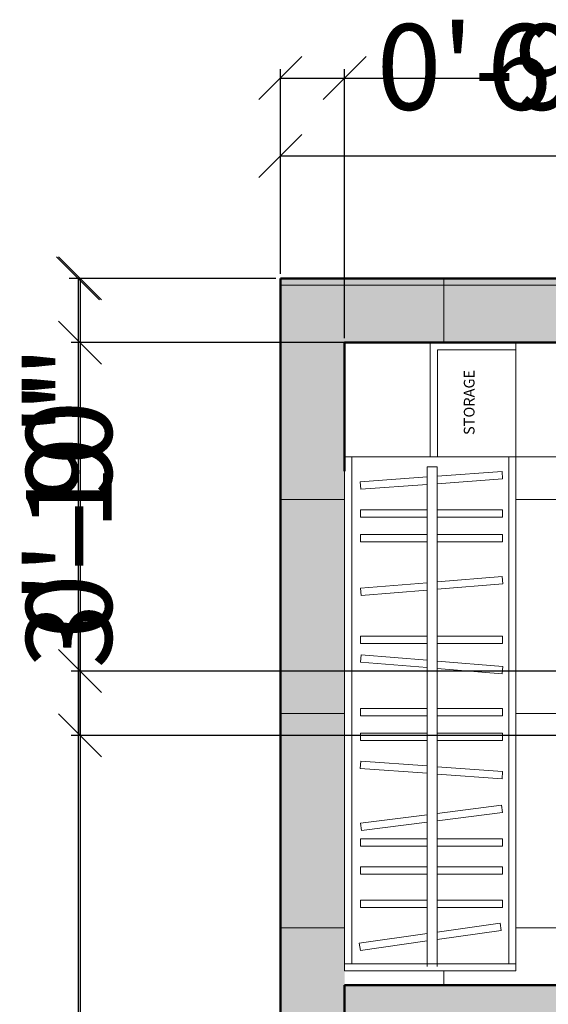
# Model space of a CAD drawing. Units: inches. Extents: x 2371 to 3019, y 129 to 700.
# Tile 4 of 14: x 2371 to 2445, y 529 to 667. Entities that reach past the tile are written whole.
import ezdxf

# ---------------------------------------------------------------- set-up
doc = ezdxf.new("R2010")
doc.units = ezdxf.units.IN
for name, color, linetype, lineweight in [('A-ANNO-DIMS', 2, 'Continuous', 18), ('A-AREA-IDEN', 7, 'Continuous', 25), ('A-FLOR-PATT', 252, 'Continuous', 13), ('A-FURN', 8, 'Continuous', 18), ('A-WALL', 7, 'Continuous', 50), ('A-WALL-PATT', 8, 'Continuous', 13)]:
    doc.layers.add(name, color=color, linetype=linetype, lineweight=lineweight)
doc.styles.get("Standard").update_dxf_attribs({"font": 'arial.ttf'})
doc.dimstyles.new('ISO-25', dxfattribs={"dimtxt": 12, "dimasz": 6, "dimexe": 1.25, "dimexo": 0.625, "dimtad": 0, "dimdec": 1, "dimlunit": 3, "dimtxsty": 'Standard', "dimblk": 'OBLIQUE', "dimblk1": 'ORIGIN2', "dimblk2": 'OBLIQUE', "dimcen": 2.5, "dimadec": 0, "dimazin": 0, "dimtfac": 1, "dimtdec": 1, "dimtmove": 0, "dimatfit": 3, "dimldrblk": 'OBLIQUE', "dimfxl": 1, "dimarcsym": 0})

# ---------------------------------------------------------------- blocks, each defined once
blk = doc.blocks.new('_Oblique')
at = {"color": 0, "linetype": 'ByBlock', "lineweight": -2}
blk.add_line((-0.5, -0.5), (0.5, 0.5), dxfattribs=at)
blk = doc.blocks.new('*D14')
at = {"layer": 'A-ANNO-DIMS', "color": 0, "lineweight": -2, "transparency": 16777216}
for p, q in [((2407.11, 631.6), (2407.11, 649.37)), ((2407.11, 648.12), (2643.63, 648.12)), ((2923.11, 648.12), (2686.58, 648.12)), ((2923.11, 631.6), (2923.11, 649.37))]:
    blk.add_line(p, q, dxfattribs=at)
at = {"layer": 'Defpoints', "color": 0, "lineweight": 25, "transparency": 16777216}
for p in [(2923.11, 648.12), (2407.11, 630.98), (2923.11, 630.98)]:
    blk.add_point(p, dxfattribs=at)
at = {"layer": 'A-ANNO-DIMS', "color": 0, "lineweight": -2, "transparency": 16777216, "xscale": 6, "yscale": 6, "zscale": 6, "rotation": 180}
blk.add_blockref('_Oblique', (2407.11, 648.12), dxfattribs=at)
at = {"layer": 'A-ANNO-DIMS', "color": 0, "lineweight": -2, "transparency": 16777216, "xscale": 6, "yscale": 6, "zscale": 6}
blk.add_blockref('_Oblique', (2923.11, 648.12), dxfattribs=at)
at = {"layer": 'A-ANNO-DIMS', "color": 0, "transparency": 16777216, "insert": (2665.11, 648.12), "char_height": 12, "width": 20.8486, "attachment_point": 5}
blk.add_mtext('43\'-0"', dxfattribs=at)
blk = doc.blocks.new('_Origin2')
at = {"color": 0, "linetype": 'ByBlock', "lineweight": -2}
blk.add_line((-0.5, 0), (-1, 0), dxfattribs=at)
for radius in [0.5, 0.25]:
    blk.add_circle((0, 0), radius, dxfattribs=at)
blk = doc.blocks.new('*D18')
at = {"layer": 'A-ANNO-DIMS', "color": 0, "lineweight": -2, "transparency": 16777216}
for p, q in [((2406.48, 630.98), (2377.53, 630.98)), ((2378.78, 630.98), (2378.78, 484.31)), ((2378.78, 294.98), (2378.78, 441.64)), ((2406.48, 294.98), (2377.53, 294.98))]:
    blk.add_line(p, q, dxfattribs=at)
at = {"layer": 'Defpoints', "color": 0, "lineweight": 25, "transparency": 16777216}
for p in [(2407.11, 630.98), (2378.78, 294.98), (2407.11, 294.98)]:
    blk.add_point(p, dxfattribs=at)
at = {"layer": 'A-ANNO-DIMS', "color": 0, "lineweight": -2, "transparency": 16777216, "xscale": 6, "yscale": 6, "zscale": 6}
for p, rotation in [((2378.78, 630.98), 90), ((2378.78, 294.98), 270)]:
    blk.add_blockref('_Oblique', p, dxfattribs=dict(at, rotation=rotation))
at = {"layer": 'A-ANNO-DIMS', "color": 0, "transparency": 16777216, "insert": (2378.78, 462.98), "char_height": 12, "attachment_point": 5, "rotation": 90}
blk.add_mtext('28\'-0"', dxfattribs=at)
blk = doc.blocks.new('*D34')
at = {"layer": 'A-ANNO-DIMS', "color": 0, "lineweight": -2, "transparency": 16777216}
for p, q in [((2407.11, 631.6), (2407.11, 660.28)), ((2416.11, 622.6), (2416.11, 660.28)), ((2407.11, 659.03), (2416.11, 659.03)), ((2416.11, 659.03), (2422.11, 659.03))]:
    blk.add_line(p, q, dxfattribs=at)
at = {"layer": 'Defpoints', "color": 0, "lineweight": 25, "transparency": 16777216}
for p in [(2416.11, 659.03), (2407.11, 630.98), (2416.11, 621.98)]:
    blk.add_point(p, dxfattribs=at)
at = {"layer": 'A-ANNO-DIMS', "color": 0, "lineweight": -2, "transparency": 16777216, "xscale": 6, "yscale": 6, "zscale": 6, "rotation": 180}
blk.add_blockref('_Oblique', (2407.11, 659.03), dxfattribs=at)
at = {"layer": 'A-ANNO-DIMS', "color": 0, "lineweight": -2, "transparency": 16777216, "xscale": 6, "yscale": 6, "zscale": 6}
blk.add_blockref('_Oblique', (2416.11, 659.03), dxfattribs=at)
at = {"layer": 'A-ANNO-DIMS', "color": 0, "transparency": 16777216, "insert": (2438.68, 659.03), "char_height": 12, "attachment_point": 5}
blk.add_mtext('0\'-9"', dxfattribs=at)
blk = doc.blocks.new('*D35')
at = {"layer": 'A-ANNO-DIMS', "color": 0, "lineweight": -2, "transparency": 16777216}
for p, q in [((2416.11, 622.6), (2416.11, 660.28)), ((2492.11, 622.6), (2492.11, 660.28)), ((2416.11, 659.03), (2437.5, 659.03)), ((2492.11, 659.03), (2470.71, 659.03))]:
    blk.add_line(p, q, dxfattribs=at)
at = {"layer": 'Defpoints', "color": 0, "lineweight": 25, "transparency": 16777216}
for p in [(2492.11, 659.03), (2416.11, 621.98), (2492.11, 621.98)]:
    blk.add_point(p, dxfattribs=at)
at = {"layer": 'A-ANNO-DIMS', "color": 0, "lineweight": -2, "transparency": 16777216, "xscale": 6, "yscale": 6, "zscale": 6, "rotation": 180}
blk.add_blockref('_Oblique', (2416.11, 659.03), dxfattribs=at)
at = {"layer": 'A-ANNO-DIMS', "color": 0, "lineweight": -2, "transparency": 16777216, "xscale": 6, "yscale": 6, "zscale": 6}
blk.add_blockref('_Oblique', (2492.11, 659.03), dxfattribs=at)
at = {"layer": 'A-ANNO-DIMS', "color": 0, "transparency": 16777216, "insert": (2454.11, 659.03), "char_height": 12, "attachment_point": 5}
blk.add_mtext('6\'-4"', dxfattribs=at)
blk = doc.blocks.new('*D60')
at = {"layer": 'A-ANNO-DIMS', "color": 0, "lineweight": -2, "transparency": 16777216}
for p, q in [((2406.48, 630.98), (2377.81, 630.98)), ((2379.06, 630.98), (2379.06, 518.81)), ((2379.06, 363.98), (2379.06, 476.14)), ((2406.48, 363.98), (2377.81, 363.98))]:
    blk.add_line(p, q, dxfattribs=at)
at = {"layer": 'Defpoints', "color": 0, "lineweight": 25, "transparency": 16777216}
for p in [(2379.06, 630.98), (2407.11, 630.98), (2407.11, 363.98)]:
    blk.add_point(p, dxfattribs=at)
at = {"layer": 'A-ANNO-DIMS', "color": 0, "lineweight": -2, "transparency": 16777216, "xscale": 6, "yscale": 6, "zscale": 6}
for p, rotation in [((2379.06, 630.98), 90), ((2379.06, 363.98), 270)]:
    blk.add_blockref('_Oblique', p, dxfattribs=dict(at, rotation=rotation))
at = {"layer": 'A-ANNO-DIMS', "color": 0, "transparency": 16777216, "insert": (2379.06, 497.48), "char_height": 12, "attachment_point": 5, "rotation": 90}
blk.add_mtext('22\'-3"', dxfattribs=at)
blk = doc.blocks.new('*D65')
at = {"layer": 'A-ANNO-DIMS', "color": 0, "lineweight": -2, "transparency": 16777216}
for p, q in [((2618.98, 621.98), (2377.81, 621.98)), ((2379.06, 621.98), (2379.06, 620.21)), ((2379.06, 575.98), (2379.06, 577.74)), ((2616.98, 575.98), (2377.81, 575.98))]:
    blk.add_line(p, q, dxfattribs=at)
at = {"layer": 'Defpoints', "color": 0, "lineweight": 25, "transparency": 16777216}
for p in [(2379.06, 621.98), (2619.61, 621.98), (2617.61, 575.98)]:
    blk.add_point(p, dxfattribs=at)
at = {"layer": 'A-ANNO-DIMS', "color": 0, "lineweight": -2, "transparency": 16777216, "xscale": 6, "yscale": 6, "zscale": 6}
for p, rotation in [((2379.06, 621.98), 90), ((2379.06, 575.98), 270)]:
    blk.add_blockref('_Oblique', p, dxfattribs=dict(at, rotation=rotation))
at = {"layer": 'A-ANNO-DIMS', "color": 0, "transparency": 16777216, "insert": (2379.06, 598.98), "char_height": 12, "attachment_point": 5, "rotation": 90}
blk.add_mtext('3\'-10"', dxfattribs=at)
blk = doc.blocks.new('*D67')
at = {"layer": 'A-ANNO-DIMS', "color": 0, "lineweight": -2, "transparency": 16777216}
for p, q in [((2379.06, 575.98), (2379.06, 581.98)), ((2616.98, 575.98), (2377.81, 575.98)), ((2379.06, 566.98), (2379.06, 575.98)), ((2616.98, 566.98), (2377.81, 566.98))]:
    blk.add_line(p, q, dxfattribs=at)
at = {"layer": 'Defpoints', "color": 0, "lineweight": 25, "transparency": 16777216}
for p in [(2379.06, 575.98), (2617.61, 575.98), (2617.61, 566.98)]:
    blk.add_point(p, dxfattribs=at)
at = {"layer": 'A-ANNO-DIMS', "color": 0, "lineweight": -2, "transparency": 16777216, "xscale": 6, "yscale": 6, "zscale": 6}
for p, rotation in [((2379.06, 575.98), 90), ((2379.06, 566.98), 270)]:
    blk.add_blockref('_Oblique', p, dxfattribs=dict(at, rotation=rotation))
at = {"layer": 'A-ANNO-DIMS', "color": 0, "transparency": 16777216, "insert": (2379.06, 598.55), "char_height": 12, "attachment_point": 5, "rotation": 90}
blk.add_mtext('0\'-9"', dxfattribs=at)

msp = doc.modelspace()

# ---------------------------------------------------------------- hatches: boundary and pattern name
at = {"layer": 'A-FLOR-PATT'}
h = msp.add_hatch(dxfattribs=at)
h.set_pattern_fill('_USER', color=256, scale=30, pattern_type=0)
h.set_pattern_definition([(0, (0, 0), (0, 30), [])])
h.paths.add_polyline_path([(2913.11, 498.98), (2827.61, 498.98), (2827.61, 531.98), (2832.11, 531.98), (2832.11, 537.98), (2833.61, 537.98), (2833.61, 605.98), (2818.35, 605.98, -1), (2796.86, 605.98), (2781.61, 605.98), (2781.61, 603.98), (2781.61, 533.98), (2757.61, 533.98), (2757.61, 531.98), (2797.61, 531.98), (2797.61, 522.98), (2757.61, 522.98), (2757.61, 516.98), (2754.59, 516.98), (2772.52, 485.76), (2771.01, 484.89), (2770.98, 484.93, -0.097552), (2757.61, 481.1), (2757.61, 422.48), (2837.61, 422.48), (2837.61, 362.48), (2757.61, 362.48), (2757.61, 303.98), (2835.86, 303.98, -0.09439), (2793.86, 311.98), (2793.86, 337.98), (2799.86, 337.98), (2799.86, 336.42), (2871.86, 336.42), (2871.86, 337.98), (2877.86, 337.98), (2877.86, 311.98, -0.09439), (2835.86, 303.98), (2913.11, 303.98), (2913.11, 383.18), (2904.11, 383.18), (2904.11, 419.18), (2913.11, 419.18)])
h.paths.add_polyline_path([(2788.88, 332.88), (2788.88, 308.88), (2764.88, 308.88), (2764.88, 332.88)], flags=16)
h.paths.add_polyline_path([(2788.4, 325.04, -1), (2774.4, 325.04, -1)], flags=0)
h.paths.add_polyline_path([(2781.4, 328.04), (2784.4, 325.04), (2781.4, 322.04), (2778.4, 325.04)], flags=0)
h.paths.add_polyline_path([(2782.4, 325.04, -1), (2780.4, 325.04, -1)], flags=0)
h.paths.add_polyline_path([(2748.61, 480.99), (2754.51, 480.98, 0.119303), (2770.98, 484.93), (2753.07, 516.1), (2754.59, 516.98), (2748.61, 516.98), (2748.61, 539.98), (2712.61, 539.98), (2665.11, 539.98, -0.09439), (2707.11, 531.98), (2707.11, 505.98), (2701.11, 505.98), (2701.11, 507.53), (2629.11, 507.53), (2629.11, 505.98), (2623.11, 505.98), (2623.11, 531.98, -0.09439), (2665.11, 539.98), (2581.61, 539.98), (2581.61, 522.98), (2581.61, 477.98, -0.131044), (2589.61, 507.98), (2615.61, 507.98), (2615.61, 501.98), (2614.05, 501.98), (2614.05, 453.98), (2615.61, 453.98), (2615.61, 447.98), (2589.61, 447.98, -0.131044), (2581.61, 477.98), (2581.61, 432.98), (2572.61, 432.98, 0.119303), (2556.14, 428.99), (2574.12, 397.85), (2572.61, 396.98), (2578.61, 396.98), (2581.61, 396.98), (2581.61, 390.98), (2748.61, 390.98)])
h.paths.add_polyline_path([(2683.1, 447.25), (2652.43, 447.25), (2652.43, 492.22), (2683.1, 492.22)], flags=16)
h.paths.add_polyline_path([(2682.1, 448.25), (2653.43, 448.25), (2653.43, 491.22), (2682.1, 491.22)], flags=0)
h.paths.add_polyline_path([(2613.58, 512.06), (2589.58, 512.06), (2589.58, 536.06), (2613.58, 536.06)], flags=16)
h.paths.add_polyline_path([(2599.1, 528.22, -1), (2613.1, 528.22, -1)], flags=0)
h.paths.add_polyline_path([(2609.1, 528.22), (2606.1, 525.22), (2603.1, 528.22), (2606.1, 531.22)], flags=0)
h.paths.add_polyline_path([(2607.1, 528.22, -1), (2605.1, 528.22, -1)], flags=0)
h.paths.add_polyline_path([(2581.61, 522.98), (2581.61, 621.98), (2572.61, 621.98), (2572.61, 522.98), (2572.61, 500.98), (2565.85, 500.98), (2565.85, 500.15), (2564.82, 500.15), (2561.16, 500.19), (2561.16, 500.17), (2560.13, 500.3), (2560.22, 500.98), (2556.38, 500.98), (2556.43, 500.22), (2555.4, 500.14), (2555.34, 500.98), (2551.07, 500.98), (2551.07, 500.15), (2550.04, 500.15), (2547.64, 500.19), (2547.64, 500.15), (2546.61, 500.15), (2541.79, 500.22), (2540.72, 500.13), (2540.65, 500.98), (2533.37, 500.98), (2533.37, 500.15), (2532.34, 500.15), (2529.13, 500.21), (2529.12, 500.13), (2528.09, 500.22), (2528.16, 500.98), (2523.23, 500.98), (2523.23, 500.15), (2522.2, 500.15), (2519.8, 500.21), (2519.8, 500.15), (2518.77, 500.15), (2514.45, 500.26), (2514.44, 500.14), (2513.41, 500.22), (2513.47, 500.98), (2509.62, 500.98), (2509.71, 500.3), (2508.69, 500.17), (2508.58, 500.98), (2505.03, 500.98), (2505.03, 500.15), (2503.99, 500.15), (2501.07, 500.29), (2501.07, 500.15), (2500.04, 500.15), (2496.44, 500.37), (2496.44, 500.15), (2495.4, 500.15), (2492.55, 500.41), (2492.18, 500.35), (2492.09, 500.98), (2486.11, 500.98), (2486.11, 524.98), (2486.11, 531.98), (2490.61, 531.98), (2490.61, 537.98), (2492.11, 537.98), (2492.11, 605.98), (2476.85, 605.98, -1), (2455.36, 605.98), (2440.11, 605.98), (2440.11, 533.98), (2416.11, 533.98), (2416.11, 605.98), (2416.11, 621.98), (2536.61, 621.98), (2536.61, 630.98), (2407.11, 630.98), (2407.11, 363.98), (2416.11, 363.98), (2416.11, 431.48), (2496.11, 431.48), (2496.11, 371.48), (2416.11, 371.48), (2416.11, 303.98), (2494.36, 303.98, -0.09439), (2452.36, 311.98), (2452.36, 337.98), (2458.36, 337.98), (2458.36, 336.42), (2530.36, 336.42), (2530.36, 337.98), (2536.36, 337.98), (2536.36, 311.98, -0.09439), (2494.36, 303.98), (2572.61, 303.98), (2572.61, 381.98), (2572.61, 396.98), (2554.61, 428.15), (2556.12, 429.03), (2556.14, 428.99, -0.119303), (2572.61, 432.98), (2578.61, 432.98), (2581.61, 432.98)])
h.paths.add_polyline_path([(2450.11, 500.98), (2444.5, 500.98), (2444.44, 500.14), (2443.41, 500.22), (2443.47, 500.98), (2439.62, 500.98), (2439.71, 500.3), (2438.69, 500.17), (2438.58, 500.98), (2435.02, 500.98), (2435.02, 500.15), (2433.99, 500.15), (2433.99, 500.98), (2431.07, 500.98), (2431.07, 500.15), (2430.04, 500.15), (2430.04, 500.98), (2426.43, 500.98), (2426.43, 500.15), (2425.4, 500.15), (2425.4, 500.98), (2423.13, 500.98), (2423.2, 500.5), (2422.18, 500.35), (2422.09, 500.98), (2416.11, 500.98), (2416.11, 524.98), (2416.11, 531.98), (2450.11, 531.98), (2450.11, 522.98)], flags=16)
h.paths.add_polyline_path([(2449.11, 501.98), (2417.11, 501.98), (2417.11, 522.98), (2417.11, 523.98), (2449.11, 523.98)], flags=0)
h.paths.add_polyline_path([(2420.7, 510.73), (2419.36, 520.07), (2420.38, 520.22), (2421.74, 510.73), (2425.4, 510.73), (2425.4, 520.07), (2426.43, 520.07), (2426.43, 510.73), (2430.04, 510.73), (2430.04, 520.07), (2431.07, 520.07), (2431.07, 510.73), (2433.99, 510.73), (2433.99, 520.07), (2435.02, 520.07), (2435.02, 510.73), (2437.35, 510.73), (2436.18, 519.93), (2437.2, 520.06), (2438.39, 510.73), (2444.17, 510.73), (2444.85, 520.08), (2445.88, 520.01), (2445.21, 510.73)], flags=0)
h.paths.add_polyline_path([(2446.94, 336.11), (2446.94, 312.11), (2422.94, 312.11), (2422.94, 336.11)], flags=16)
h.paths.add_polyline_path([(2446.46, 328.27, -1), (2432.46, 328.27, -1)], flags=0)
h.paths.add_polyline_path([(2439.46, 331.27), (2442.46, 328.27), (2439.46, 325.27), (2436.46, 328.27)], flags=0)
h.paths.add_polyline_path([(2440.46, 328.27, -1), (2438.46, 328.27, -1)], flags=0)
h.paths.add_polyline_path([(2816, 444.88), (2866.87, 444.88), (2866.87, 463.54), (2816, 463.54)], flags=24)
h.paths.add_polyline_path([(2794.21, 558.3), (2833.34, 558.3), (2833.34, 576.96), (2794.21, 576.96)], flags=24)
h.paths.add_polyline_path([(2651.69, 411.53), (2711.04, 411.53), (2711.04, 430.19), (2651.69, 430.19)], flags=24)
h.paths.add_polyline_path([(2494.09, 444.88), (2544.97, 444.88), (2544.97, 463.54), (2494.09, 463.54)], flags=24)
h.paths.add_polyline_path([(2444.55, 565.02), (2483.69, 565.02), (2483.69, 583.68), (2444.55, 583.68)], flags=24)
h = msp.add_hatch(dxfattribs=at)
h.set_pattern_fill('_USER', color=256, scale=30, angle=90, pattern_type=0)
h.set_pattern_definition([(90, (0, 0), (-30, 2e-15), [])])
h.paths.add_polyline_path([(2913.11, 498.98), (2827.61, 498.98), (2827.61, 531.98), (2832.11, 531.98), (2832.11, 537.98), (2833.61, 537.98), (2833.61, 605.98), (2818.35, 605.98, -1), (2796.86, 605.98), (2781.61, 605.98), (2781.61, 603.98), (2781.61, 533.98), (2757.61, 533.98), (2757.61, 531.98), (2797.61, 531.98), (2797.61, 522.98), (2757.61, 522.98), (2757.61, 516.98), (2754.59, 516.98), (2772.52, 485.76), (2771.01, 484.89), (2770.98, 484.93, -0.097552), (2757.61, 481.1), (2757.61, 422.48), (2837.61, 422.48), (2837.61, 362.48), (2757.61, 362.48), (2757.61, 303.98), (2835.86, 303.98, -0.09439), (2793.86, 311.98), (2793.86, 337.98), (2799.86, 337.98), (2799.86, 336.42), (2871.86, 336.42), (2871.86, 337.98), (2877.86, 337.98), (2877.86, 311.98, -0.09439), (2835.86, 303.98), (2913.11, 303.98), (2913.11, 383.18), (2904.11, 383.18), (2904.11, 419.18), (2913.11, 419.18)])
h.paths.add_polyline_path([(2788.88, 332.88), (2788.88, 308.88), (2764.88, 308.88), (2764.88, 332.88)], flags=16)
h.paths.add_polyline_path([(2788.4, 325.04, -1), (2774.4, 325.04, -1)], flags=0)
h.paths.add_polyline_path([(2781.4, 328.04), (2784.4, 325.04), (2781.4, 322.04), (2778.4, 325.04)], flags=0)
h.paths.add_polyline_path([(2782.4, 325.04, -1), (2780.4, 325.04, -1)], flags=0)
h.paths.add_polyline_path([(2748.61, 480.99), (2754.51, 480.98, 0.119303), (2770.98, 484.93), (2753.07, 516.1), (2754.59, 516.98), (2748.61, 516.98), (2748.61, 539.98), (2712.61, 539.98), (2665.11, 539.98, -0.09439), (2707.11, 531.98), (2707.11, 505.98), (2701.11, 505.98), (2701.11, 507.53), (2629.11, 507.53), (2629.11, 505.98), (2623.11, 505.98), (2623.11, 531.98, -0.09439), (2665.11, 539.98), (2581.61, 539.98), (2581.61, 522.98), (2581.61, 477.98, -0.131044), (2589.61, 507.98), (2615.61, 507.98), (2615.61, 501.98), (2614.05, 501.98), (2614.05, 453.98), (2615.61, 453.98), (2615.61, 447.98), (2589.61, 447.98, -0.131044), (2581.61, 477.98), (2581.61, 432.98), (2572.61, 432.98, 0.119303), (2556.14, 428.99), (2574.12, 397.85), (2572.61, 396.98), (2578.61, 396.98), (2581.61, 396.98), (2581.61, 390.98), (2748.61, 390.98)])
h.paths.add_polyline_path([(2683.1, 447.25), (2652.43, 447.25), (2652.43, 492.22), (2683.1, 492.22)], flags=16)
h.paths.add_polyline_path([(2682.1, 448.25), (2653.43, 448.25), (2653.43, 491.22), (2682.1, 491.22)], flags=0)
h.paths.add_polyline_path([(2613.58, 512.06), (2589.58, 512.06), (2589.58, 536.06), (2613.58, 536.06)], flags=16)
h.paths.add_polyline_path([(2599.1, 528.22, -1), (2613.1, 528.22, -1)], flags=0)
h.paths.add_polyline_path([(2609.1, 528.22), (2606.1, 525.22), (2603.1, 528.22), (2606.1, 531.22)], flags=0)
h.paths.add_polyline_path([(2607.1, 528.22, -1), (2605.1, 528.22, -1)], flags=0)
h.paths.add_polyline_path([(2581.61, 522.98), (2581.61, 621.98), (2572.61, 621.98), (2572.61, 522.98), (2572.61, 500.98), (2565.85, 500.98), (2565.85, 500.15), (2564.82, 500.15), (2561.16, 500.19), (2561.16, 500.17), (2560.13, 500.3), (2560.22, 500.98), (2556.38, 500.98), (2556.43, 500.22), (2555.4, 500.14), (2555.34, 500.98), (2551.07, 500.98), (2551.07, 500.15), (2550.04, 500.15), (2547.64, 500.19), (2547.64, 500.15), (2546.61, 500.15), (2541.79, 500.22), (2540.72, 500.13), (2540.65, 500.98), (2533.37, 500.98), (2533.37, 500.15), (2532.34, 500.15), (2529.13, 500.21), (2529.12, 500.13), (2528.09, 500.22), (2528.16, 500.98), (2523.23, 500.98), (2523.23, 500.15), (2522.2, 500.15), (2519.8, 500.21), (2519.8, 500.15), (2518.77, 500.15), (2514.45, 500.26), (2514.44, 500.14), (2513.41, 500.22), (2513.47, 500.98), (2509.62, 500.98), (2509.71, 500.3), (2508.69, 500.17), (2508.58, 500.98), (2505.03, 500.98), (2505.03, 500.15), (2503.99, 500.15), (2501.07, 500.29), (2501.07, 500.15), (2500.04, 500.15), (2496.44, 500.37), (2496.44, 500.15), (2495.4, 500.15), (2492.55, 500.41), (2492.18, 500.35), (2492.09, 500.98), (2486.11, 500.98), (2486.11, 524.98), (2486.11, 531.98), (2490.61, 531.98), (2490.61, 537.98), (2492.11, 537.98), (2492.11, 605.98), (2476.85, 605.98, -1), (2455.36, 605.98), (2440.11, 605.98), (2440.11, 533.98), (2416.11, 533.98), (2416.11, 605.98), (2416.11, 621.98), (2536.61, 621.98), (2536.61, 630.98), (2407.11, 630.98), (2407.11, 363.98), (2416.11, 363.98), (2416.11, 431.48), (2496.11, 431.48), (2496.11, 371.48), (2416.11, 371.48), (2416.11, 303.98), (2494.36, 303.98, -0.09439), (2452.36, 311.98), (2452.36, 337.98), (2458.36, 337.98), (2458.36, 336.42), (2530.36, 336.42), (2530.36, 337.98), (2536.36, 337.98), (2536.36, 311.98, -0.09439), (2494.36, 303.98), (2572.61, 303.98), (2572.61, 381.98), (2572.61, 396.98), (2554.61, 428.15), (2556.12, 429.03), (2556.14, 428.99, -0.119303), (2572.61, 432.98), (2578.61, 432.98), (2581.61, 432.98)])
h.paths.add_polyline_path([(2450.11, 500.98), (2444.5, 500.98), (2444.44, 500.14), (2443.41, 500.22), (2443.47, 500.98), (2439.62, 500.98), (2439.71, 500.3), (2438.69, 500.17), (2438.58, 500.98), (2435.02, 500.98), (2435.02, 500.15), (2433.99, 500.15), (2433.99, 500.98), (2431.07, 500.98), (2431.07, 500.15), (2430.04, 500.15), (2430.04, 500.98), (2426.43, 500.98), (2426.43, 500.15), (2425.4, 500.15), (2425.4, 500.98), (2423.13, 500.98), (2423.2, 500.5), (2422.18, 500.35), (2422.09, 500.98), (2416.11, 500.98), (2416.11, 524.98), (2416.11, 531.98), (2450.11, 531.98), (2450.11, 522.98)], flags=16)
h.paths.add_polyline_path([(2449.11, 501.98), (2417.11, 501.98), (2417.11, 522.98), (2417.11, 523.98), (2449.11, 523.98)], flags=0)
h.paths.add_polyline_path([(2420.7, 510.73), (2419.36, 520.07), (2420.38, 520.22), (2421.74, 510.73), (2425.4, 510.73), (2425.4, 520.07), (2426.43, 520.07), (2426.43, 510.73), (2430.04, 510.73), (2430.04, 520.07), (2431.07, 520.07), (2431.07, 510.73), (2433.99, 510.73), (2433.99, 520.07), (2435.02, 520.07), (2435.02, 510.73), (2437.35, 510.73), (2436.18, 519.93), (2437.2, 520.06), (2438.39, 510.73), (2444.17, 510.73), (2444.85, 520.08), (2445.88, 520.01), (2445.21, 510.73)], flags=0)
h.paths.add_polyline_path([(2446.94, 336.11), (2446.94, 312.11), (2422.94, 312.11), (2422.94, 336.11)], flags=16)
h.paths.add_polyline_path([(2446.46, 328.27, -1), (2432.46, 328.27, -1)], flags=0)
h.paths.add_polyline_path([(2439.46, 331.27), (2442.46, 328.27), (2439.46, 325.27), (2436.46, 328.27)], flags=0)
h.paths.add_polyline_path([(2440.46, 328.27, -1), (2438.46, 328.27, -1)], flags=0)
h.paths.add_polyline_path([(2816, 444.88), (2866.87, 444.88), (2866.87, 463.54), (2816, 463.54)], flags=24)
h.paths.add_polyline_path([(2794.21, 558.3), (2833.34, 558.3), (2833.34, 576.96), (2794.21, 576.96)], flags=24)
h.paths.add_polyline_path([(2651.69, 411.53), (2711.04, 411.53), (2711.04, 430.19), (2651.69, 430.19)], flags=24)
h.paths.add_polyline_path([(2494.09, 444.88), (2544.97, 444.88), (2544.97, 463.54), (2494.09, 463.54)], flags=24)
h.paths.add_polyline_path([(2444.55, 565.02), (2483.69, 565.02), (2483.69, 583.68), (2444.55, 583.68)], flags=24)
at = {"layer": 'A-WALL-PATT'}
h = msp.add_hatch(color=256, dxfattribs=at)
h.dxf.hatch_style = 1
h.paths.add_polyline_path([(2536.61, 630.98), (2407.11, 630.98), (2407.11, 363.98), (2416.11, 363.98), (2416.11, 498.98), (2416.11, 522.98), (2416.11, 531.98), (2416.11, 603.98), (2416.11, 621.98), (2536.61, 621.98)])
h.paths.add_polyline_path([(2630.98, 630.98), (2560.61, 630.98), (2560.61, 621.98), (2630.98, 621.98)])
h.paths.add_polyline_path([(2878.11, 630.98), (2699.23, 630.98), (2699.23, 621.98), (2878.11, 621.98)])
h.paths.add_polyline_path([(2496.61, 621.98), (2492.11, 621.98), (2492.11, 569.98), (2496.61, 569.98)], flags=17)
h.paths.add_polyline_path([(2581.61, 621.98), (2572.61, 621.98), (2572.61, 522.98), (2572.61, 498.98), (2572.61, 432.98), (2578.61, 432.98), (2581.61, 432.98), (2581.61, 522.98)])
h.paths.add_polyline_path([(2572.61, 531.98), (2486.11, 531.98), (2486.11, 522.98), (2572.61, 522.98)])
h.paths.add_polyline_path([(2450.11, 531.98), (2440.11, 531.98), (2416.11, 531.98), (2416.11, 522.98), (2450.11, 522.98)], flags=17)
h.paths.add_polyline_path([(2416.11, 315.98), (2407.11, 315.98), (2407.11, 294.98), (2458.11, 294.98), (2458.11, 303.98), (2416.11, 303.98)])
h.paths.add_polyline_path([(2757.61, 303.98), (2530.61, 303.98), (2530.61, 294.98), (2757.61, 294.98)])
h.paths.add_polyline_path([(2581.61, 381.98), (2605.61, 381.98), (2617.61, 381.98), (2617.61, 390.98), (2581.61, 390.98), (2581.61, 396.98), (2572.61, 396.98), (2572.61, 381.98), (2572.61, 303.98), (2581.61, 303.98)])
h.paths.add_polyline_path([(2757.61, 480.98), (2748.61, 480.98), (2748.61, 381.98), (2748.61, 303.98), (2757.61, 303.98), (2757.61, 381.98), (2757.61, 422.48)])
h.paths.add_polyline_path([(2797.61, 531.98), (2757.61, 531.98), (2757.61, 603.98), (2757.61, 621.98), (2748.61, 621.98), (2748.61, 516.99), (2754.59, 516.98), (2757.61, 516.98), (2757.61, 522.98), (2797.61, 522.98)])
h.paths.add_polyline_path([(2913.11, 531.98), (2827.61, 531.98), (2827.61, 522.98), (2913.11, 522.98)])
h.paths.add_polyline_path([(2923.11, 630.98), (2902.11, 630.98), (2902.11, 621.98), (2914.11, 621.98), (2914.11, 363.98), (2923.11, 363.98)])
h.paths.add_polyline_path([(2923.11, 315.98), (2914.11, 315.98), (2914.11, 303.98), (2866.11, 303.98), (2866.11, 294.98), (2923.11, 294.98)])
h.paths.add_polyline_path([(2793.61, 303.98), (2757.61, 303.98), (2757.61, 294.98), (2793.61, 294.98)])

# ---------------------------------------------------------------- linework, layer by layer
at = {"layer": 'A-FURN'}
for p, q in [((2428.11, 605.98), (2428.11, 621.98)), ((2440.11, 621.98), (2440.11, 603.98)), ((2429.11, 605.98), (2429.11, 620.98)), ((2429.11, 620.98), (2440.11, 620.98)), ((2492.11, 605.98), (2440.11, 605.98)), ((2427.66, 604.59), (2427.66, 534.65)), ((2429.06, 534.65), (2429.06, 604.59)), ((2427.66, 549.09), (2427.66, 534.59)), ((2429.06, 534.59), (2429.06, 549.09)), ((2440.11, 534.98), (2416.11, 534.98))]:
    msp.add_line(p, q, dxfattribs=at)
msp.add_lwpolyline([(2440.11, 605.98), (2440.11, 533.98), (2416.11, 533.98), (2416.11, 605.98)], close=True, dxfattribs=at)
for points in [[(2417.11, 605.98), (2417.11, 534.98), (2439.11, 534.98), (2439.11, 605.98)], [(2439.11, 604.98), (2439.11, 534.98), (2417.11, 534.98), (2417.11, 604.98)], [(2427.66, 604.59), (2429.06, 604.59)], [(2427.66, 602.12), (2418.38, 601.45), (2418.31, 602.48), (2427.66, 603.16)], [(2429.06, 603.26), (2438.17, 603.92), (2438.25, 602.89)], [(2438.25, 602.89), (2429.06, 602.22)], [(2427.66, 597.53), (2418.32, 597.53), (2418.32, 598.56), (2427.66, 598.56)], [(2429.06, 598.56), (2438.24, 598.56), (2438.24, 597.53)], [(2438.24, 597.53), (2429.06, 597.53)], [(2427.66, 594.09), (2418.32, 594.09), (2418.32, 595.13), (2427.66, 595.13)], [(2429.06, 595.13), (2438.24, 595.13), (2438.24, 594.09)], [(2438.24, 594.09), (2429.06, 594.09)], [(2429.06, 588.48), (2438.17, 589.24), (2438.26, 588.21)], [(2427.66, 587.33), (2418.41, 586.56), (2418.33, 587.58), (2427.66, 588.36)], [(2438.26, 588.21), (2429.06, 587.44)], [(2427.66, 580.86), (2418.32, 580.86), (2418.32, 579.83), (2427.66, 579.83)], [(2438.24, 580.86), (2429.06, 580.86)], [(2429.06, 579.83), (2438.24, 579.83), (2438.24, 580.86)], [(2427.66, 577.49), (2418.41, 578.26), (2418.33, 577.23), (2427.66, 576.46)], [(2438.26, 576.61), (2429.06, 577.37)], [(2429.06, 576.34), (2438.17, 575.58), (2438.26, 576.61)], [(2427.66, 570.72), (2418.32, 570.72), (2418.32, 569.69), (2427.66, 569.69)], [(2438.24, 570.72), (2429.06, 570.72)], [(2429.06, 569.69), (2438.24, 569.69), (2438.24, 570.72)], [(2427.66, 567.29), (2418.32, 567.29), (2418.32, 566.26), (2427.66, 566.26)], [(2438.24, 567.29), (2429.06, 567.29)], [(2429.06, 566.26), (2438.24, 566.26), (2438.24, 567.29)], [(2427.66, 562.69), (2418.38, 563.37), (2418.31, 562.34), (2427.66, 561.66)], [(2438.25, 561.93), (2429.06, 562.59)], [(2429.06, 561.56), (2438.17, 560.9), (2438.25, 561.93)], [(2438.09, 557.2), (2429.06, 556.05)], [(2429.06, 555.01), (2438.22, 556.17), (2438.09, 557.2)], [(2427.66, 555.87), (2418.33, 554.69), (2418.46, 553.67), (2427.66, 554.84)], [(2427.66, 552.51), (2418.32, 552.51), (2418.32, 551.48), (2427.66, 551.48)], [(2438.24, 552.51), (2429.06, 552.51)], [(2429.06, 551.48), (2438.24, 551.48), (2438.24, 552.51)], [(2427.66, 548.56), (2418.32, 548.56), (2418.32, 547.53), (2427.66, 547.53)], [(2438.24, 548.56), (2429.06, 548.56)], [(2429.06, 547.53), (2438.24, 547.53), (2438.24, 548.56)], [(2427.66, 543.92), (2418.32, 543.92), (2418.32, 542.89), (2427.66, 542.89)], [(2438.24, 543.92), (2429.06, 543.92)], [(2429.06, 542.89), (2438.24, 542.89), (2438.24, 543.92)], [(2437.89, 540.69), (2429.06, 539.43)], [(2429.06, 538.39), (2438.04, 539.67), (2437.89, 540.69)], [(2427.66, 539.23), (2418.17, 537.87), (2418.32, 536.85), (2427.66, 538.19)]]:
    msp.add_lwpolyline(points, dxfattribs=at)
at = {"layer": 'A-WALL'}
for p, q in [((2407.11, 630.98), (2407.11, 294.98)), ((2536.61, 630.98), (2407.11, 630.98)), ((2416.11, 621.98), (2416.11, 603.98)), ((2536.61, 621.98), (2416.11, 621.98)), ((2416.11, 531.98), (2416.11, 522.98)), ((2450.11, 531.98), (2416.11, 531.98))]:
    msp.add_line(p, q, dxfattribs=at)

# ---------------------------------------------------------------- texts
at = {"layer": 'A-AREA-IDEN', "insert": (2432.81, 609.04), "char_height": 1.5, "attachment_point": 1, "rotation": 90}
msp.add_mtext_dynamic_manual_height_columns('STORAGE', width=1.7945, gutter_width=12.5, heights=[0], dxfattribs=at)

# ---------------------------------------------------------------- dimensions: what is measured, and where the dimension line sits
at = {"layer": 'A-ANNO-DIMS'}
for base, p1, p2, picture, middle in [((2416.11, 659.03), (2407.11, 630.98), (2416.11, 621.98), '*D34', (2438.68, 659.03)), ((2492.11, 659.03), (2416.11, 621.98), (2492.11, 621.98), '*D35', (2454.11, 659.03))]:
    dim = msp.add_linear_dim(base=base, p1=p1, p2=p2, dimstyle='ISO-25', override={"dimdec": 1, "dimlfac": 1, "dimrnd": 0, "dimzin": 1, "dimdsep": 46, "dimlunit": 4, "dimfrac": 2}, dxfattribs=at)
    dim.commit()
    dim.dimension.update_dxf_attribs({"geometry": picture, "text_midpoint": middle})
dim = msp.add_linear_dim(base=(2923.11, 648.12), p1=(2407.11, 630.98), p2=(2923.11, 630.98), text='43\'-0"', dimstyle='ISO-25', override={"dimclrd": 0, "dimclre": 0, "dimclrt": 0}, dxfattribs=at)
dim.commit()
dim.dimension.update_dxf_attribs({"geometry": '*D14', "text_midpoint": (2665.11, 648.12)})
dim = msp.add_linear_dim(base=(2378.78, 294.98), p1=(2407.11, 630.98), p2=(2407.11, 294.98), angle=90, text='28\'-0"', dimstyle='ISO-25', override={"dimclrd": 0, "dimclre": 0, "dimclrt": 0}, dxfattribs=at)
dim.commit()
dim.dimension.update_dxf_attribs({"geometry": '*D18', "text_midpoint": (2378.78, 462.98)})
for base, p1, p2, picture, middle in [((2379.06, 630.98), (2407.11, 363.98), (2407.11, 630.98), '*D60', (2379.06, 497.48)), ((2379.06, 621.98), (2617.61, 575.98), (2619.61, 621.98), '*D65', (2379.06, 598.98)), ((2379.06, 575.98), (2617.61, 566.98), (2617.61, 575.98), '*D67', (2379.06, 598.55))]:
    dim = msp.add_linear_dim(base=base, p1=p1, p2=p2, angle=90, dimstyle='ISO-25', override={"dimdec": 1, "dimlfac": 1, "dimrnd": 0, "dimzin": 1, "dimdsep": 46, "dimlunit": 4, "dimfrac": 2}, dxfattribs=at)
    dim.commit()
    dim.dimension.update_dxf_attribs({"geometry": picture, "text_midpoint": middle})

doc.saveas('drawing.dxf')
